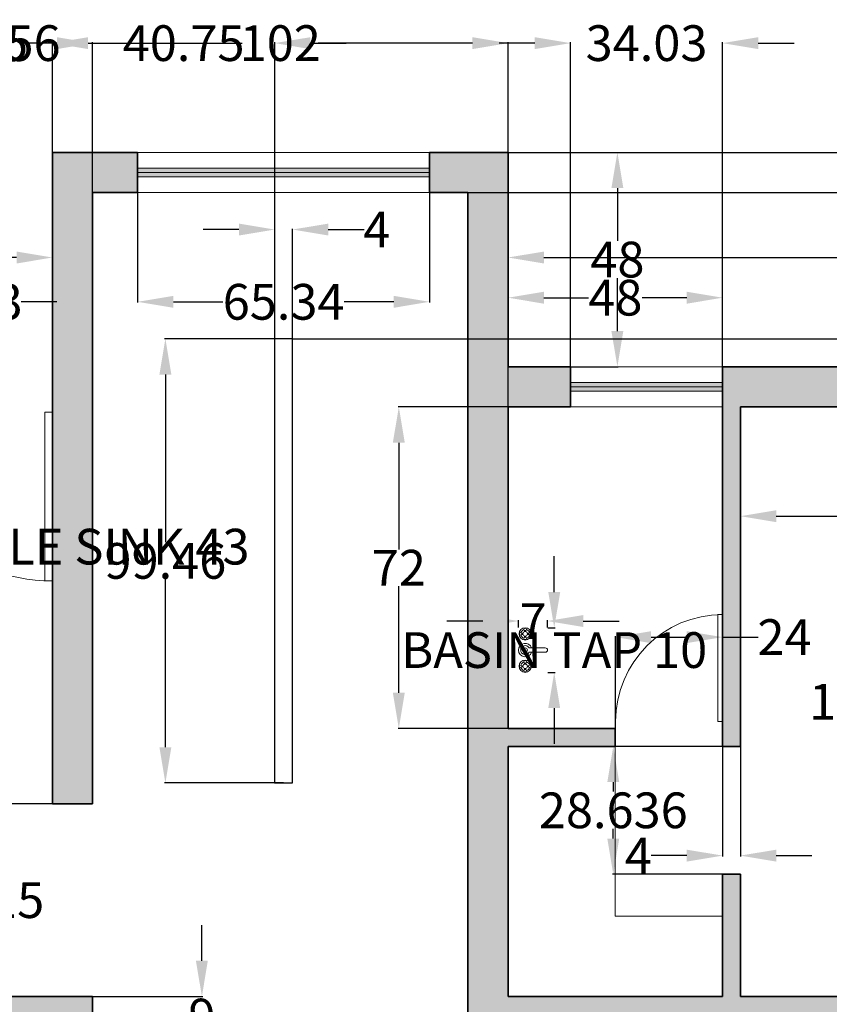
# Model space of a CAD drawing. Units: inches. Extents: x -52 to 678, y 23 to 685.
# Tile 8 of 11: x 249 to 431, y 334 to 555. Entities that reach past the tile are written whole.
import ezdxf

# ---------------------------------------------------------------- set-up
doc = ezdxf.new("R2010")
doc.units = ezdxf.units.IN
doc.header["$MEASUREMENT"] = 0
for name, color, linetype, lineweight in [('A-ANNO-DIMS', 2, 'Continuous', 18), ('A-DOOR', 3, 'Continuous', 18), ('A-FLOR-CASE', 8, 'Continuous', 18), ('A-FLOR-FIXT', 9, 'Continuous', 18), ('A-FLOR-STRS', 7, 'Continuous', 25), ('A-GLAZ', 4, 'Continuous', 18), ('A-WALL', 7, 'Continuous', 35)]:
    doc.layers.add(name, color=color, linetype=linetype, lineweight=lineweight)
doc.layers.add('A-GLAZ-PATT', color=18, linetype='Continuous', lineweight=13, true_color=0x000000)
doc.layers.add('A-WALL-PATT', color=18, linetype='Continuous', lineweight=13, true_color=0x000000)
doc.styles.get("Standard").update_dxf_attribs({"font": 'arial.ttf'})
doc.dimstyles.get("Standard").update_dxf_attribs({"dimtxt": 8, "dimasz": 8, "dimexe": 0.18, "dimexo": 0.0625, "dimgap": 0.09, "dimtad": 0, "dimtih": 1, "dimtoh": 1, "dimdec": 0, "dimzin": 0, "dimdsep": 46, "dimlunit": 3, "dimtxsty": 'Standard', "dimcen": 0.09, "dimadec": 0, "dimazin": 0, "dimtfac": 1, "dimtdec": 0, "dimtofl": 0, "dimtmove": 0, "dimatfit": 3, "dimfxl": 1, "dimtolj": 1, "dimtzin": 0, "dimarcsym": 0})

# ---------------------------------------------------------------- blocks, each defined once
blk = doc.blocks.new('Faucet - Bathroom top')
for p, q in [((-4.107, 0.125), (-4.375, 0.125)), ((-3.75, 0.4788), (-3.75, 0.75)), ((-3.5, 0.482), (-3.5, 0.75)), ((-3.1461, 0.125), (-2.875, 0.125)), ((3.143, 0.125), (2.875, 0.125)), ((3.5, 0.4788), (3.5, 0.75)), ((3.75, 0.482), (3.75, 0.75)), ((4.1039, 0.125), (4.375, 0.125)), ((-4.1039, -0.125), (-4.375, -0.125)), ((-3.75, -0.4821), (-3.75, -0.75)), ((-3.5, -0.4789), (-3.5, -0.75)), ((-3.143, -0.125), (-2.875, -0.125)), ((-0.5, -0.8639), (-0.5, -4.5)), ((0.5, -4.5), (0.5, -0.8631)), ((3.1461, -0.125), (2.875, -0.125)), ((3.5, -0.4821), (3.5, -0.75)), ((3.75, -0.4789), (3.75, -0.75)), ((4.107, -0.125), (4.375, -0.125))]:
    blk.add_line(p, q)
for centre, radius in [((-3.625, 0), 1.375), ((-4.625, 0), 0.2795), ((-3.625, 0), 0.5), ((-3.625, 1), 0.2795), ((-2.625, 0), 0.2795), ((0, 0), 0.5), ((3.625, 0), 1.375), ((2.625, 0), 0.2795), ((3.625, 0), 0.5), ((3.625, 1), 0.2795), ((4.625, 0), 0.2795), ((-3.625, -1), 0.2795), ((3.625, -1), 0.2795)]:
    blk.add_circle(centre, radius)
for centre, radius, start, end in [((-3.625, 0), 1, 105.2407, 164.2093), ((-3.625, 0), 1, 16.44125, 74.07887), ((0, 0), 1.5, 289.6514, 250.3603), ((0, 0), 1, 300.3431, 239.7554), ((3.625, 0), 1, 106.12, 164.0884), ((3.625, 0), 1, 16.23422, 73.90469), ((-3.625, 0), 1, 196.2342, 253.9047), ((-3.625, 0), 1, 286.12, 344.0884), ((3.625, 0), 1, 196.4413, 254.0789), ((3.625, 0), 1, 285.2407, 344.2093), ((0, -4.5), 0.5, 180, 0)]:
    blk.add_arc(centre, radius, start, end)
blk = doc.blocks.new('*U16')
for p, q in [((-40, 0), (-40, 6)), ((0, 0), (0, 6))]:
    blk.add_line(p, q)
blk.add_lwpolyline([(0, 0), (0, -40), (-1.75, -40), (-1.75, 0)], close=True)
blk.add_arc((0, 0), 40, 180, 270)
blk = doc.blocks.new('*U15')
for p, q in [((0, 0), (0, -6)), ((-40, 0), (-40, -6))]:
    blk.add_line(p, q)
blk.add_lwpolyline([(0, 0), (0, 40), (-1.75, 40), (-1.75, 0)], close=True)
blk.add_arc((0, 0), 40, 90, 180)
blk = doc.blocks.new('*D29')
at = {"layer": 'A-ANNO-DIMS', "color": 0, "lineweight": -2, "transparency": 16777216}
for p, q in [((163.02, 443.19), (163.02, 436.67)), ((205.67, 443.19), (205.67, 436.67)), ((171.02, 436.85), (197.67, 436.85)), ((205.67, 436.85), (213.67, 436.85))]:
    blk.add_line(p, q, dxfattribs=at)
at = {"layer": 'A-ANNO-DIMS', "color": 0, "transparency": 16777216}
for points in [[(171.02, 438.19), (171.02, 435.52), (163.02, 436.85)], [(197.67, 438.19), (197.67, 435.52), (205.67, 436.85)]]:
    blk.add_solid(points, dxfattribs=at)
at = {"layer": 'Defpoints', "color": 0, "transparency": 16777216}
for p in [(163.02, 443.25), (205.67, 443.25), (205.67, 436.85)]:
    blk.add_point(p, dxfattribs=at)
at = {"layer": 'A-ANNO-DIMS', "color": 0, "transparency": 16777216, "insert": (258.41, 436.85), "char_height": 8, "attachment_point": 5}
blk.add_mtext('\\A1;DOUBLE SINK 43', dxfattribs=at)
blk = doc.blocks.new('*D35')
at = {"layer": 'A-ANNO-DIMS', "color": 0, "lineweight": -2, "transparency": 16777216}
for p, q in [((368.93, 426.69), (368.93, 434.69)), ((367.5, 418.69), (369.11, 418.69)), ((367.5, 408.69), (369.11, 408.69)), ((368.93, 400.69), (368.93, 392.69))]:
    blk.add_line(p, q, dxfattribs=at)
at = {"layer": 'A-ANNO-DIMS', "color": 0, "transparency": 16777216}
for points in [[(367.6, 426.69), (370.27, 426.69), (368.93, 418.69)], [(367.6, 400.69), (370.27, 400.69), (368.93, 408.69)]]:
    blk.add_solid(points, dxfattribs=at)
at = {"layer": 'Defpoints', "color": 0, "transparency": 16777216}
for p in [(367.43, 418.69), (368.93, 418.69), (367.43, 408.69)]:
    blk.add_point(p, dxfattribs=at)
at = {"layer": 'A-ANNO-DIMS', "color": 0, "transparency": 16777216, "insert": (368.93, 413.69), "char_height": 8, "attachment_point": 5}
blk.add_mtext('\\A1;BASIN TAP 10', dxfattribs=at)
blk = doc.blocks.new('*D36')
at = {"layer": 'A-ANNO-DIMS', "color": 0, "lineweight": -2, "transparency": 16777216}
for p, q in [((352.93, 420.19), (344.93, 420.19)), ((360.93, 418.76), (360.93, 420.37)), ((367.43, 418.76), (367.43, 420.37)), ((375.43, 420.19), (383.43, 420.19))]:
    blk.add_line(p, q, dxfattribs=at)
at = {"layer": 'A-ANNO-DIMS', "color": 0, "transparency": 16777216}
for points in [[(352.93, 421.53), (352.93, 418.86), (360.93, 420.19)], [(375.43, 421.53), (375.43, 418.86), (367.43, 420.19)]]:
    blk.add_solid(points, dxfattribs=at)
at = {"layer": 'Defpoints', "color": 0, "transparency": 16777216}
for p in [(360.93, 420.19), (360.93, 418.69), (367.43, 418.69)]:
    blk.add_point(p, dxfattribs=at)
at = {"layer": 'A-ANNO-DIMS', "color": 0, "transparency": 16777216, "insert": (364.18, 420.19), "char_height": 8, "attachment_point": 5}
blk.add_mtext('\\A1;7', dxfattribs=at)
blk = doc.blocks.new('*D40')
at = {"layer": 'A-ANNO-DIMS', "color": 0, "lineweight": -2, "transparency": 16777216}
for p, q in [((358.67, 525.13), (600.25, 525.13)), ((600.07, 517.13), (600.07, 293.23)), ((600.07, 61.13), (600.07, 285.02)), ((575.67, 53.13), (600.25, 53.13))]:
    blk.add_line(p, q, dxfattribs=at)
at = {"layer": 'A-ANNO-DIMS', "color": 0, "transparency": 16777216}
for points in [[(598.73, 517.13), (601.4, 517.13), (600.07, 525.13)], [(598.73, 61.13), (601.4, 61.13), (600.07, 53.13)]]:
    blk.add_solid(points, dxfattribs=at)
at = {"layer": 'Defpoints', "color": 0, "transparency": 16777216}
for p in [(358.61, 525.13), (600.07, 525.13), (575.61, 53.13)]:
    blk.add_point(p, dxfattribs=at)
at = {"layer": 'A-ANNO-DIMS', "color": 0, "transparency": 16777216, "insert": (600.07, 289.13), "char_height": 8, "attachment_point": 5}
blk.add_mtext('\\A1;472', dxfattribs=at)
blk = doc.blocks.new('*D41')
at = {"layer": 'A-ANNO-DIMS', "color": 0, "lineweight": -2, "transparency": 16777216}
for p, q in [((91.61, 477.19), (91.61, 501.77)), ((99.61, 501.59), (165.52, 501.59)), ((248.61, 501.59), (182.69, 501.59)), ((256.61, 477.19), (256.61, 501.77))]:
    blk.add_line(p, q, dxfattribs=at)
at = {"layer": 'A-ANNO-DIMS', "color": 0, "transparency": 16777216}
for points in [[(99.61, 502.92), (99.61, 500.25), (91.61, 501.59)], [(248.61, 502.92), (248.61, 500.25), (256.61, 501.59)]]:
    blk.add_solid(points, dxfattribs=at)
at = {"layer": 'Defpoints', "color": 0, "transparency": 16777216}
for p in [(256.61, 501.59), (91.61, 477.13), (256.61, 477.13)]:
    blk.add_point(p, dxfattribs=at)
at = {"layer": 'A-ANNO-DIMS', "color": 0, "transparency": 16777216, "insert": (174.11, 501.59), "char_height": 8, "attachment_point": 5}
blk.add_mtext('\\A1;165', dxfattribs=at)
blk = doc.blocks.new('*D42')
at = {"layer": 'A-ANNO-DIMS', "color": 0, "lineweight": -2, "transparency": 16777216}
for p, q in [((256.61, 525.19), (256.61, 549.77)), ((264.61, 549.59), (299.1, 549.59)), ((350.61, 549.59), (316.12, 549.59)), ((358.61, 525.19), (358.61, 549.77))]:
    blk.add_line(p, q, dxfattribs=at)
at = {"layer": 'A-ANNO-DIMS', "color": 0, "transparency": 16777216}
for points in [[(264.61, 550.92), (264.61, 548.25), (256.61, 549.59)], [(350.61, 550.92), (350.61, 548.25), (358.61, 549.59)]]:
    blk.add_solid(points, dxfattribs=at)
at = {"layer": 'Defpoints', "color": 0, "transparency": 16777216}
for p in [(358.61, 549.59), (256.61, 525.13), (358.61, 525.13)]:
    blk.add_point(p, dxfattribs=at)
at = {"layer": 'A-ANNO-DIMS', "color": 0, "transparency": 16777216, "insert": (307.61, 549.59), "char_height": 8, "attachment_point": 5}
blk.add_mtext('\\A1;102', dxfattribs=at)
blk = doc.blocks.new('*D43')
at = {"layer": 'A-ANNO-DIMS', "color": 0, "lineweight": -2, "transparency": 16777216}
for p, q in [((358.61, 477.19), (358.61, 501.77)), ((366.61, 501.59), (458.11, 501.59)), ((567.61, 501.59), (476.1, 501.59)), ((575.61, 477.19), (575.61, 501.77))]:
    blk.add_line(p, q, dxfattribs=at)
at = {"layer": 'A-ANNO-DIMS', "color": 0, "transparency": 16777216}
for points in [[(366.61, 502.92), (366.61, 500.25), (358.61, 501.59)], [(567.61, 502.92), (567.61, 500.25), (575.61, 501.59)]]:
    blk.add_solid(points, dxfattribs=at)
at = {"layer": 'Defpoints', "color": 0, "transparency": 16777216}
for p in [(575.61, 501.59), (358.61, 477.13), (575.61, 477.13)]:
    blk.add_point(p, dxfattribs=at)
at = {"layer": 'A-ANNO-DIMS', "color": 0, "transparency": 16777216, "insert": (467.11, 501.59), "char_height": 8, "attachment_point": 5}
blk.add_mtext('\\A1;217', dxfattribs=at)
blk = doc.blocks.new('*D44')
at = {"layer": 'A-ANNO-DIMS', "color": 0, "lineweight": -2, "transparency": 16777216}
for p, q in [((358.67, 525.13), (383.25, 525.13)), ((383.07, 517.13), (383.07, 505.3)), ((383.07, 485.13), (383.07, 496.95)), ((358.67, 477.13), (383.25, 477.13))]:
    blk.add_line(p, q, dxfattribs=at)
at = {"layer": 'A-ANNO-DIMS', "color": 0, "transparency": 16777216}
for points in [[(381.73, 517.13), (384.4, 517.13), (383.07, 525.13)], [(381.73, 485.13), (384.4, 485.13), (383.07, 477.13)]]:
    blk.add_solid(points, dxfattribs=at)
at = {"layer": 'Defpoints', "color": 0, "transparency": 16777216}
for p in [(358.61, 525.13), (358.61, 477.13), (383.07, 477.13)]:
    blk.add_point(p, dxfattribs=at)
at = {"layer": 'A-ANNO-DIMS', "color": 0, "transparency": 16777216, "insert": (383.07, 501.13), "char_height": 8, "attachment_point": 5}
blk.add_mtext('\\A1;48', dxfattribs=at)
blk = doc.blocks.new('*D53')
at = {"layer": 'A-ANNO-DIMS', "color": 0, "lineweight": -2, "transparency": 16777216}
for p, q in [((358.61, 468.19), (358.61, 492.77)), ((366.61, 492.59), (376.62, 492.59)), ((398.61, 492.59), (388.59, 492.59)), ((406.61, 468.19), (406.61, 492.77))]:
    blk.add_line(p, q, dxfattribs=at)
at = {"layer": 'A-ANNO-DIMS', "color": 0, "transparency": 16777216}
for points in [[(366.61, 493.92), (366.61, 491.25), (358.61, 492.59)], [(398.61, 493.92), (398.61, 491.25), (406.61, 492.59)]]:
    blk.add_solid(points, dxfattribs=at)
at = {"layer": 'Defpoints', "color": 0, "transparency": 16777216}
for p in [(406.61, 492.59), (358.61, 468.13), (406.61, 468.13)]:
    blk.add_point(p, dxfattribs=at)
at = {"layer": 'A-ANNO-DIMS', "color": 0, "transparency": 16777216, "insert": (382.61, 492.59), "char_height": 8, "attachment_point": 5}
blk.add_mtext('\\A1;48', dxfattribs=at)
blk = doc.blocks.new('*D54')
at = {"layer": 'A-ANNO-DIMS', "color": 0, "lineweight": -2, "transparency": 16777216}
for p, q in [((358.54, 468.13), (333.97, 468.13)), ((334.15, 460.13), (334.15, 436.23)), ((334.15, 404.13), (334.15, 428.02)), ((358.54, 396.13), (333.97, 396.13))]:
    blk.add_line(p, q, dxfattribs=at)
at = {"layer": 'A-ANNO-DIMS', "color": 0, "transparency": 16777216}
for points in [[(332.81, 460.13), (335.48, 460.13), (334.15, 468.13)], [(332.81, 404.13), (335.48, 404.13), (334.15, 396.13)]]:
    blk.add_solid(points, dxfattribs=at)
at = {"layer": 'Defpoints', "color": 0, "transparency": 16777216}
for p in [(334.15, 468.13), (358.61, 468.13), (358.61, 396.13)]:
    blk.add_point(p, dxfattribs=at)
at = {"layer": 'A-ANNO-DIMS', "color": 0, "transparency": 16777216, "insert": (334.15, 432.13), "char_height": 8, "attachment_point": 5}
blk.add_mtext('\\A1;72', dxfattribs=at)
blk = doc.blocks.new('*D57')
at = {"layer": 'A-ANNO-DIMS', "color": 0, "lineweight": -2, "transparency": 16777216}
for p, q in [((410.61, 468.06), (410.61, 443.49)), ((566.61, 468.06), (566.61, 443.49)), ((418.61, 443.67), (480.06, 443.67)), ((558.61, 443.67), (497.15, 443.67))]:
    blk.add_line(p, q, dxfattribs=at)
at = {"layer": 'A-ANNO-DIMS', "color": 0, "transparency": 16777216}
for points in [[(418.61, 445), (418.61, 442.33), (410.61, 443.67)], [(558.61, 445), (558.61, 442.33), (566.61, 443.67)]]:
    blk.add_solid(points, dxfattribs=at)
at = {"layer": 'Defpoints', "color": 0, "transparency": 16777216}
for p in [(410.61, 468.13), (566.61, 468.13), (410.61, 443.67)]:
    blk.add_point(p, dxfattribs=at)
at = {"layer": 'A-ANNO-DIMS', "color": 0, "transparency": 16777216, "insert": (488.61, 443.67), "char_height": 8, "attachment_point": 5}
blk.add_mtext('\\A1;156', dxfattribs=at)
blk = doc.blocks.new('*D58')
at = {"layer": 'A-ANNO-DIMS', "color": 0, "lineweight": -2, "transparency": 16777216}
for p, q in [((410.67, 468.13), (435.25, 468.13)), ((435.07, 460.13), (435.07, 406.3)), ((435.07, 344.13), (435.07, 397.95)), ((410.67, 336.13), (435.25, 336.13))]:
    blk.add_line(p, q, dxfattribs=at)
at = {"layer": 'A-ANNO-DIMS', "color": 0, "transparency": 16777216}
for points in [[(433.73, 460.13), (436.4, 460.13), (435.07, 468.13)], [(433.73, 344.13), (436.4, 344.13), (435.07, 336.13)]]:
    blk.add_solid(points, dxfattribs=at)
at = {"layer": 'Defpoints', "color": 0, "transparency": 16777216}
for p in [(410.61, 468.13), (410.61, 336.13), (435.07, 336.13)]:
    blk.add_point(p, dxfattribs=at)
at = {"layer": 'A-ANNO-DIMS', "color": 0, "transparency": 16777216, "insert": (435.07, 402.13), "char_height": 8, "attachment_point": 5}
blk.add_mtext('\\A1;132', dxfattribs=at)
blk = doc.blocks.new('*D59')
at = {"layer": 'A-ANNO-DIMS', "color": 0, "lineweight": -2, "transparency": 16777216}
for p, q in [((290.07, 344.13), (290.07, 352.13)), ((265.67, 336.13), (290.25, 336.13)), ((265.67, 327.13), (290.25, 327.13)), ((290.07, 319.13), (290.07, 311.13))]:
    blk.add_line(p, q, dxfattribs=at)
at = {"layer": 'A-ANNO-DIMS', "color": 0, "transparency": 16777216}
for points in [[(288.73, 344.13), (291.4, 344.13), (290.07, 336.13)], [(288.73, 319.13), (291.4, 319.13), (290.07, 327.13)]]:
    blk.add_solid(points, dxfattribs=at)
at = {"layer": 'Defpoints', "color": 0, "transparency": 16777216}
for p in [(265.61, 336.13), (265.61, 327.13), (290.07, 327.13)]:
    blk.add_point(p, dxfattribs=at)
at = {"layer": 'A-ANNO-DIMS', "color": 0, "transparency": 16777216, "insert": (290.07, 331.63), "char_height": 8, "attachment_point": 5}
blk.add_mtext('\\A1;9', dxfattribs=at)
blk = doc.blocks.new('*D60')
at = {"layer": 'A-ANNO-DIMS', "color": 0, "lineweight": -2, "transparency": 16777216}
for p, q in [((406.61, 392.06), (406.61, 367.49)), ((410.61, 392.06), (410.61, 367.49)), ((398.61, 367.67), (390.61, 367.67)), ((418.61, 367.67), (426.61, 367.67))]:
    blk.add_line(p, q, dxfattribs=at)
at = {"layer": 'A-ANNO-DIMS', "color": 0, "transparency": 16777216}
for points in [[(398.61, 369), (398.61, 366.33), (406.61, 367.67)], [(418.61, 369), (418.61, 366.33), (410.61, 367.67)]]:
    blk.add_solid(points, dxfattribs=at)
at = {"layer": 'Defpoints', "color": 0, "transparency": 16777216}
for p in [(406.61, 392.13), (410.61, 392.13), (406.61, 367.67)]:
    blk.add_point(p, dxfattribs=at)
at = {"layer": 'A-ANNO-DIMS', "color": 0, "transparency": 16777216, "insert": (387.75, 367.67), "char_height": 8, "attachment_point": 5}
blk.add_mtext('\\A1;4', dxfattribs=at)
blk = doc.blocks.new('*D61')
at = {"layer": 'A-ANNO-DIMS', "color": 0, "lineweight": -2, "transparency": 16777216}
for p, q in [((210.46, 549.59), (202.46, 549.59)), ((218.46, 477.19), (218.46, 549.77)), ((256.61, 477.19), (256.61, 549.77)), ((264.61, 549.59), (272.61, 549.59))]:
    blk.add_line(p, q, dxfattribs=at)
at = {"layer": 'A-ANNO-DIMS', "color": 0, "transparency": 16777216}
for points in [[(210.46, 550.92), (210.46, 548.25), (218.46, 549.59)], [(264.61, 550.92), (264.61, 548.25), (256.61, 549.59)]]:
    blk.add_solid(points, dxfattribs=at)
at = {"layer": 'Defpoints', "color": 0, "transparency": 16777216}
for p in [(256.61, 549.59), (218.46, 477.13), (256.61, 477.13)]:
    blk.add_point(p, dxfattribs=at)
at = {"layer": 'A-ANNO-DIMS', "color": 0, "transparency": 16777216, "insert": (237.53, 549.59), "char_height": 8, "attachment_point": 5}
blk.add_mtext('\\A1;38.15', dxfattribs=at)
blk = doc.blocks.new('*D64')
at = {"layer": 'A-ANNO-DIMS', "color": 0, "lineweight": -2, "transparency": 16777216}
for p, q in [((275.69, 516.06), (275.69, 491.49)), ((341.02, 516.06), (341.02, 491.49)), ((283.69, 491.67), (294.76, 491.67)), ((333.02, 491.67), (321.95, 491.67))]:
    blk.add_line(p, q, dxfattribs=at)
at = {"layer": 'A-ANNO-DIMS', "color": 0, "transparency": 16777216}
for points in [[(283.69, 493), (283.69, 490.33), (275.69, 491.67)], [(333.02, 493), (333.02, 490.33), (341.02, 491.67)]]:
    blk.add_solid(points, dxfattribs=at)
at = {"layer": 'Defpoints', "color": 0, "transparency": 16777216}
for p in [(275.69, 516.13), (341.02, 516.13), (275.69, 491.67)]:
    blk.add_point(p, dxfattribs=at)
at = {"layer": 'A-ANNO-DIMS', "color": 0, "transparency": 16777216, "insert": (308.36, 491.67), "char_height": 8, "attachment_point": 5}
blk.add_mtext('\\A1;65.34', dxfattribs=at)
blk = doc.blocks.new('*D65')
at = {"layer": 'A-ANNO-DIMS', "color": 0, "lineweight": -2, "transparency": 16777216}
for p, q in [((265.61, 516.06), (265.61, 491.49)), ((275.69, 516.06), (275.69, 491.49)), ((257.61, 491.67), (249.61, 491.67)), ((283.69, 491.67), (291.69, 491.67))]:
    blk.add_line(p, q, dxfattribs=at)
at = {"layer": 'A-ANNO-DIMS', "color": 0, "transparency": 16777216}
for points in [[(257.61, 493), (257.61, 490.33), (265.61, 491.67)], [(283.69, 493), (283.69, 490.33), (275.69, 491.67)]]:
    blk.add_solid(points, dxfattribs=at)
at = {"layer": 'Defpoints', "color": 0, "transparency": 16777216}
for p in [(265.61, 516.13), (275.69, 516.13), (265.61, 491.67)]:
    blk.add_point(p, dxfattribs=at)
at = {"layer": 'A-ANNO-DIMS', "color": 0, "transparency": 16777216, "insert": (233.29, 491.67), "char_height": 8, "attachment_point": 5}
blk.add_mtext('\\A1;10.083', dxfattribs=at)
blk = doc.blocks.new('*D68')
at = {"layer": 'A-ANNO-DIMS', "color": 0, "lineweight": -2, "transparency": 16777216}
for p, q in [((364.58, 549.59), (356.58, 549.59)), ((372.58, 477.19), (372.58, 549.77)), ((406.61, 477.19), (406.61, 549.77)), ((414.61, 549.59), (422.61, 549.59))]:
    blk.add_line(p, q, dxfattribs=at)
at = {"layer": 'A-ANNO-DIMS', "color": 0, "transparency": 16777216}
for points in [[(364.58, 550.92), (364.58, 548.25), (372.58, 549.59)], [(414.61, 550.92), (414.61, 548.25), (406.61, 549.59)]]:
    blk.add_solid(points, dxfattribs=at)
at = {"layer": 'Defpoints', "color": 0, "transparency": 16777216}
for p in [(406.61, 549.59), (372.58, 477.13), (406.61, 477.13)]:
    blk.add_point(p, dxfattribs=at)
at = {"layer": 'A-ANNO-DIMS', "color": 0, "transparency": 16777216, "insert": (389.59, 549.59), "char_height": 8, "attachment_point": 5}
blk.add_mtext('\\A1;34.03', dxfattribs=at)
blk = doc.blocks.new('*D81')
at = {"layer": 'A-ANNO-DIMS', "color": 0, "lineweight": -2, "transparency": 16777216}
for p, q in [((306.29, 483.39), (281.72, 483.39)), ((281.9, 475.39), (281.9, 437.84)), ((281.9, 391.93), (281.9, 429.49)), ((306.29, 383.93), (281.72, 383.93))]:
    blk.add_line(p, q, dxfattribs=at)
at = {"layer": 'A-ANNO-DIMS', "color": 0, "transparency": 16777216}
for points in [[(280.56, 475.39), (283.23, 475.39), (281.9, 483.39)], [(280.56, 391.93), (283.23, 391.93), (281.9, 383.93)]]:
    blk.add_solid(points, dxfattribs=at)
at = {"layer": 'Defpoints', "color": 0, "transparency": 16777216}
for p in [(281.9, 483.39), (306.36, 483.39), (306.36, 383.93)]:
    blk.add_point(p, dxfattribs=at)
at = {"layer": 'A-ANNO-DIMS', "color": 0, "transparency": 16777216, "insert": (281.9, 433.66), "char_height": 8, "attachment_point": 5}
blk.add_mtext('\\A1;99.46', dxfattribs=at)
blk = doc.blocks.new('*D82')
at = {"layer": 'A-ANNO-DIMS', "color": 0, "lineweight": -2, "transparency": 16777216}
for p, q in [((298.36, 507.85), (290.36, 507.85)), ((306.36, 483.45), (306.36, 508.03)), ((310.36, 483.45), (310.36, 508.03)), ((318.36, 507.85), (326.36, 507.85))]:
    blk.add_line(p, q, dxfattribs=at)
at = {"layer": 'A-ANNO-DIMS', "color": 0, "transparency": 16777216}
for points in [[(298.36, 509.18), (298.36, 506.52), (306.36, 507.85)], [(318.36, 509.18), (318.36, 506.52), (310.36, 507.85)]]:
    blk.add_solid(points, dxfattribs=at)
at = {"layer": 'Defpoints', "color": 0, "transparency": 16777216}
for p in [(310.36, 507.85), (306.36, 483.39), (310.36, 483.39)]:
    blk.add_point(p, dxfattribs=at)
at = {"layer": 'A-ANNO-DIMS', "color": 0, "transparency": 16777216, "insert": (329.21, 507.85), "char_height": 8, "attachment_point": 5}
blk.add_mtext('\\A1;4', dxfattribs=at)
blk = doc.blocks.new('*D83')
at = {"layer": 'A-ANNO-DIMS', "color": 0, "lineweight": -2, "transparency": 16777216}
for p, q in [((257.61, 549.59), (249.61, 549.59)), ((265.61, 379.34), (265.61, 549.77)), ((306.36, 383.99), (306.36, 549.77)), ((314.36, 549.59), (322.36, 549.59))]:
    blk.add_line(p, q, dxfattribs=at)
at = {"layer": 'A-ANNO-DIMS', "color": 0, "transparency": 16777216}
for points in [[(257.61, 550.92), (257.61, 548.25), (265.61, 549.59)], [(314.36, 550.92), (314.36, 548.25), (306.36, 549.59)]]:
    blk.add_solid(points, dxfattribs=at)
at = {"layer": 'Defpoints', "color": 0, "transparency": 16777216}
for p in [(306.36, 549.59), (306.36, 383.93), (265.61, 379.27)]:
    blk.add_point(p, dxfattribs=at)
at = {"layer": 'A-ANNO-DIMS', "color": 0, "transparency": 16777216, "insert": (285.98, 549.59), "char_height": 8, "attachment_point": 5}
blk.add_mtext('\\A1;40.75', dxfattribs=at)
blk = doc.blocks.new('*D84')
at = {"layer": 'A-ANNO-DIMS', "color": 0, "lineweight": -2, "transparency": 16777216}
for p, q in [((265.54, 379.27), (240.97, 379.27)), ((241.15, 371.27), (241.15, 361.88)), ((241.15, 344.13), (241.15, 353.52)), ((265.54, 336.13), (240.97, 336.13))]:
    blk.add_line(p, q, dxfattribs=at)
at = {"layer": 'A-ANNO-DIMS', "color": 0, "transparency": 16777216}
for points in [[(239.81, 371.27), (242.48, 371.27), (241.15, 379.27)], [(239.81, 344.13), (242.48, 344.13), (241.15, 336.13)]]:
    blk.add_solid(points, dxfattribs=at)
at = {"layer": 'Defpoints', "color": 0, "transparency": 16777216}
for p in [(241.15, 379.27), (265.61, 379.27), (265.61, 336.13)]:
    blk.add_point(p, dxfattribs=at)
at = {"layer": 'A-ANNO-DIMS', "color": 0, "transparency": 16777216, "insert": (241.15, 357.7), "char_height": 8, "attachment_point": 5}
blk.add_mtext('\\A1;43.15', dxfattribs=at)
blk = doc.blocks.new('*D85')
at = {"layer": 'A-ANNO-DIMS', "color": 0, "lineweight": -2, "transparency": 16777216}
for p, q in [((349.67, 516.13), (600.25, 516.13)), ((600.07, 508.13), (600.07, 503.94)), ((600.07, 491.39), (600.07, 495.58)), ((310.42, 483.39), (600.25, 483.39))]:
    blk.add_line(p, q, dxfattribs=at)
at = {"layer": 'A-ANNO-DIMS', "color": 0, "transparency": 16777216}
for points in [[(598.73, 508.13), (601.4, 508.13), (600.07, 516.13)], [(598.73, 491.39), (601.4, 491.39), (600.07, 483.39)]]:
    blk.add_solid(points, dxfattribs=at)
at = {"layer": 'Defpoints', "color": 0, "transparency": 16777216}
for p in [(349.61, 516.13), (600.07, 516.13), (310.36, 483.39)]:
    blk.add_point(p, dxfattribs=at)
at = {"layer": 'A-ANNO-DIMS', "color": 0, "transparency": 16777216, "insert": (600.07, 499.76), "char_height": 8, "attachment_point": 5}
blk.add_mtext('\\A1;32.736', dxfattribs=at)
blk = doc.blocks.new('*D86')
at = {"layer": 'A-ANNO-DIMS', "color": 0, "lineweight": -2, "transparency": 16777216}
for p, q in [((382.61, 392.19), (382.61, 416.77)), ((406.61, 392.19), (406.61, 416.77)), ((390.61, 416.59), (398.61, 416.59)), ((406.61, 416.59), (414.61, 416.59))]:
    blk.add_line(p, q, dxfattribs=at)
at = {"layer": 'A-ANNO-DIMS', "color": 0, "transparency": 16777216}
for points in [[(390.61, 417.92), (390.61, 415.25), (382.61, 416.59)], [(398.61, 417.92), (398.61, 415.25), (406.61, 416.59)]]:
    blk.add_solid(points, dxfattribs=at)
at = {"layer": 'Defpoints', "color": 0, "transparency": 16777216}
for p in [(406.61, 416.59), (382.61, 392.13), (406.61, 392.13)]:
    blk.add_point(p, dxfattribs=at)
at = {"layer": 'A-ANNO-DIMS', "color": 0, "transparency": 16777216, "insert": (420.48, 416.59), "char_height": 8, "attachment_point": 5}
blk.add_mtext('\\A1;24', dxfattribs=at)
blk = doc.blocks.new('*D87')
at = {"layer": 'A-ANNO-DIMS', "color": 0, "lineweight": -2, "transparency": 16777216}
for p, q in [((406.54, 392.13), (381.97, 392.13)), ((382.15, 384.13), (382.15, 381.99)), ((382.15, 371.49), (382.15, 373.63)), ((406.54, 363.49), (381.97, 363.49))]:
    blk.add_line(p, q, dxfattribs=at)
at = {"layer": 'A-ANNO-DIMS', "color": 0, "transparency": 16777216}
for points in [[(380.81, 384.13), (383.48, 384.13), (382.15, 392.13)], [(380.81, 371.49), (383.48, 371.49), (382.15, 363.49)]]:
    blk.add_solid(points, dxfattribs=at)
at = {"layer": 'Defpoints', "color": 0, "transparency": 16777216}
for p in [(382.15, 392.13), (406.61, 392.13), (406.61, 363.49)]:
    blk.add_point(p, dxfattribs=at)
at = {"layer": 'A-ANNO-DIMS', "color": 0, "transparency": 16777216, "insert": (382.15, 377.81), "char_height": 8, "attachment_point": 5}
blk.add_mtext('\\A1;28.636', dxfattribs=at)
blk = doc.blocks.new('*D103')
at = {"layer": 'A-ANNO-DIMS', "color": 0, "lineweight": -2, "transparency": 16777216}
for p, q in [((197.61, 266.24), (197.61, 549.77)), ((205.61, 549.59), (209.46, 549.59)), ((217.46, 271.45), (217.46, 549.77)), ((217.46, 549.59), (225.46, 549.59))]:
    blk.add_line(p, q, dxfattribs=at)
at = {"layer": 'A-ANNO-DIMS', "color": 0, "transparency": 16777216}
for points in [[(205.61, 550.92), (205.61, 548.25), (197.61, 549.59)], [(209.46, 550.92), (209.46, 548.25), (217.46, 549.59)]]:
    blk.add_solid(points, dxfattribs=at)
at = {"layer": 'Defpoints', "color": 0, "transparency": 16777216}
for p in [(217.46, 549.59), (217.46, 271.39), (197.61, 266.17)]:
    blk.add_point(p, dxfattribs=at)
at = {"layer": 'A-ANNO-DIMS', "color": 0, "transparency": 16777216, "insert": (241.78, 549.59), "char_height": 8, "attachment_point": 5}
blk.add_mtext('\\A1;19.856', dxfattribs=at)

msp = doc.modelspace()

# ---------------------------------------------------------------- hatches: boundary and pattern name
at = {"layer": 'A-GLAZ-PATT'}
h = msp.add_hatch(color=256, dxfattribs=at)
h.dxf.hatch_style = 1
h.paths.add_polyline_path([(275.688, 521.6267), (275.688, 520.6267), (341.0247, 520.6267), (341.0247, 521.6267)])
h = msp.add_hatch(color=256, dxfattribs=at)
h.dxf.hatch_style = 1
h.paths.add_polyline_path([(341.0247, 519.6267), (341.0247, 520.6267), (275.688, 520.6267), (275.688, 519.6267)])
h = msp.add_hatch(color=256, dxfattribs=at)
h.dxf.hatch_style = 1
h.paths.add_polyline_path([(406.6053, 472.6267), (406.6053, 473.6267), (372.5751, 473.6267), (372.5751, 472.6267)])
h = msp.add_hatch(color=256, dxfattribs=at)
h.dxf.hatch_style = 1
h.paths.add_polyline_path([(372.5751, 472.6267), (372.5751, 471.6267), (406.6053, 471.6267), (406.6053, 472.6267)])
at = {"layer": 'A-WALL-PATT'}
h = msp.add_hatch(color=256, dxfattribs=at)
h.dxf.hatch_style = 1
h.paths.add_polyline_path([(265.6053, 516.1267), (275.688, 516.1267), (275.688, 525.1267), (256.6053, 525.1267), (256.6053, 477.1267), (256.6053, 468.1267), (256.6053, 379.2738), (265.6053, 379.2738)])
h = msp.add_hatch(color=256, dxfattribs=at)
h.dxf.hatch_style = 1
h.paths.add_polyline_path([(349.6053, 340.107), (349.6053, 327.1267), (410.6053, 327.1267), (434.6053, 327.1267), (434.6053, 336.1267), (410.6053, 336.1267), (410.6053, 340.107), (410.6053, 363.4905), (406.6053, 363.4905), (406.6053, 340.107), (406.6053, 336.1267), (358.6053, 336.1267), (358.6053, 340.107), (358.6053, 392.1267), (382.6053, 392.1267), (382.6053, 396.1267), (358.6053, 396.1267), (358.6053, 468.1267), (372.5751, 468.1267), (372.5751, 477.1267), (358.6053, 477.1267), (358.6053, 525.1267), (341.0247, 525.1267), (341.0247, 516.1267), (349.6053, 516.1267)])
h = msp.add_hatch(color=256, dxfattribs=at)
h.dxf.hatch_style = 1
h.paths.add_polyline_path([(410.6053, 477.1267), (406.6053, 477.1267), (406.6053, 392.1267), (410.6053, 392.1267), (410.6053, 468.1267), (454.1942, 468.1267), (454.1942, 477.1267)])
h = msp.add_hatch(color=256, dxfattribs=at)
h.dxf.hatch_style = 1
h.paths.add_polyline_path([(265.6053, 327.1267), (265.6053, 336.1267), (170.301, 336.1267), (170.301, 327.1267)])

# ---------------------------------------------------------------- linework, layer by layer
at = {"layer": 'A-FLOR-CASE'}
for p, q in [((382.6053, 392.1267), (382.6053, 354.0872)), ((382.6053, 354.0872), (406.6053, 354.0872))]:
    msp.add_line(p, q, dxfattribs=at)
at = {"layer": 'A-FLOR-STRS'}
for p, q in [((310.3563, 483.3905), (306.3563, 483.3905)), ((306.3563, 483.3905), (306.3563, 383.9324)), ((310.3563, 383.9324), (310.3563, 483.3905)), ((308.3563, 383.9324), (306.3563, 383.9324)), ((306.3563, 383.9324), (310.3563, 383.9324))]:
    msp.add_line(p, q, dxfattribs=at)
at = {"layer": 'A-GLAZ'}
for p, q in [((275.688, 525.1267), (341.0247, 525.1267)), ((275.688, 521.6267), (341.0247, 521.6267)), ((275.688, 520.6267), (341.0247, 520.6267)), ((275.688, 519.6267), (341.0247, 519.6267)), ((275.688, 516.1267), (341.0247, 516.1267)), ((372.5751, 477.1267), (406.6053, 477.1267)), ((372.5751, 473.6267), (406.6053, 473.6267)), ((372.5751, 472.6267), (406.6053, 472.6267)), ((372.5751, 471.6267), (406.6053, 471.6267)), ((372.5751, 468.1267), (406.6053, 468.1267))]:
    msp.add_line(p, q, dxfattribs=at)
at = {"layer": 'A-WALL'}
for p, q in [((256.6053, 525.1267), (275.688, 525.1267)), ((256.6053, 525.1267), (256.6053, 477.1267)), ((275.688, 525.1267), (256.6053, 525.1267)), ((275.688, 516.1267), (275.688, 525.1267)), ((358.6053, 525.1267), (341.0247, 525.1267)), ((341.0247, 516.1267), (341.0247, 525.1267)), ((341.0247, 525.1267), (358.6053, 525.1267)), ((358.6053, 525.1267), (358.6053, 477.1267)), ((265.6053, 516.1267), (265.6053, 379.2738)), ((275.688, 516.1267), (265.6053, 516.1267)), ((349.6053, 516.1267), (341.0247, 516.1267)), ((349.6053, 516.1267), (349.6053, 340.107)), ((256.6053, 468.1267), (256.6053, 477.1267)), ((372.5751, 477.1267), (358.6053, 477.1267)), ((372.5751, 468.1267), (372.5751, 477.1267)), ((406.6053, 477.1267), (406.6053, 392.1267)), ((410.6053, 477.1267), (406.6053, 477.1267)), ((410.6053, 477.1267), (454.1942, 477.1267)), ((256.6053, 468.1267), (256.6053, 379.2738)), ((372.5751, 468.1267), (358.6053, 468.1267)), ((358.6053, 468.1267), (358.6053, 396.1267)), ((410.6053, 468.1267), (410.6053, 392.1267)), ((410.6053, 468.1267), (454.1942, 468.1267)), ((382.6053, 396.1267), (358.6053, 396.1267)), ((382.6053, 396.1267), (382.6053, 392.1267)), ((382.6053, 392.1267), (358.6053, 392.1267)), ((358.6053, 392.1267), (358.6053, 340.107)), ((410.6053, 392.1267), (406.6053, 392.1267)), ((265.6053, 379.2738), (256.6053, 379.2738)), ((406.6053, 363.4905), (410.6053, 363.4905)), ((406.6053, 363.4905), (406.6053, 340.107)), ((410.6053, 363.4905), (410.6053, 340.107)), ((349.6053, 340.107), (349.6053, 327.1267)), ((358.6053, 336.1267), (358.6053, 340.107)), ((406.6053, 340.107), (406.6053, 336.1267)), ((410.6053, 340.107), (410.6053, 336.1267)), ((170.301, 336.1267), (265.6053, 336.1267)), ((265.6053, 336.1267), (265.6053, 327.1267)), ((406.6053, 336.1267), (358.6053, 336.1267)), ((410.6053, 336.1267), (434.6053, 336.1267))]:
    msp.add_line(p, q, dxfattribs=at)

# ---------------------------------------------------------------- block references
at = {"layer": 'A-DOOR'}
for name, p, xscale, yscale, zscale in [('*U16', (256.6053, 466.957), 0.9449538553603543, 0.9449538553603543, 0.9449538553603543), ('*U15', (406.6053, 397.7156), 0.59813756145571, 0.59813756145571, 0.59813756145571)]:
    msp.add_blockref(name, p, dxfattribs=dict(at, xscale=xscale, yscale=yscale, zscale=zscale))
at = {"layer": 'A-FLOR-FIXT', "rotation": 90}
msp.add_blockref('Faucet - Bathroom top', (362.4344, 413.693), dxfattribs=at)

# ---------------------------------------------------------------- dimensions: what is measured, and where the dimension line sits
at = {"layer": 'A-ANNO-DIMS'}
for base, p1, p2, override, picture, middle in [((217.4609, 549.5867), (197.6053, 266.1726), (217.4609, 271.3879), {"dimdec": 3, "dimlfac": 1, "dimrnd": 0, "dimzin": 0, "dimdsep": 46, "dimlunit": 2}, '*D103', (241.7774, 549.5867)), ((256.6053, 549.5867), (218.4552, 477.1267), (256.6053, 477.1267), {"dimdec": 2, "dimlfac": 1, "dimrnd": 0, "dimzin": 0, "dimdsep": 46, "dimlunit": 2}, '*D61', (237.5302, 549.5867)), ((306.3563, 549.5867), (265.6053, 379.2738), (306.3563, 383.9324), {"dimdec": 2, "dimlfac": 1, "dimrnd": 0, "dimzin": 0, "dimdsep": 46, "dimlunit": 2}, '*D83', (285.9808, 549.5867)), ((358.6053, 549.5867), (256.6053, 525.1267), (358.6053, 525.1267), {"dimdec": 0, "dimlfac": 1, "dimrnd": 0, "dimzin": 0, "dimdsep": 46, "dimlunit": 2}, '*D42', (307.6053, 549.5867)), ((406.6053, 549.5867), (372.5751, 477.1267), (406.6053, 477.1267), {"dimdec": 2, "dimlfac": 1, "dimrnd": 0, "dimzin": 0, "dimdsep": 46, "dimlunit": 2}, '*D68', (389.5902, 549.5867)), ((310.3563, 507.8505), (306.3563, 483.3905), (310.3563, 483.3905), {"dimdec": 0, "dimlfac": 1, "dimrnd": 0, "dimzin": 0, "dimdsep": 46, "dimlunit": 2}, '*D82', (329.213, 507.8505)), ((575.6053, 501.5867), (358.6053, 477.1267), (575.6053, 477.1267), {"dimdec": 0, "dimlfac": 1, "dimrnd": 0, "dimzin": 0, "dimdsep": 46, "dimlunit": 2}, '*D43', (467.1053, 501.5867)), ((406.6053, 492.5867), (358.6053, 468.1267), (406.6053, 468.1267), {"dimdec": 0, "dimlfac": 1, "dimrnd": 0, "dimzin": 0, "dimdsep": 46, "dimlunit": 2}, '*D53', (382.6053, 492.5867)), ((406.6053, 416.5867), (382.6053, 392.1267), (406.6053, 392.1267), {"dimdec": 0, "dimlfac": 1, "dimrnd": 0, "dimzin": 0, "dimdsep": 46, "dimlunit": 2}, '*D86', (420.477, 416.5867))]:
    dim = msp.add_linear_dim(base=base, p1=p1, p2=p2, dimstyle='Standard', override=override, dxfattribs=at)
    dim.commit()
    dim.dimension.update_dxf_attribs({"geometry": picture, "text_midpoint": middle})
for base, p1, p2, angle, override, picture, middle in [((600.0653, 525.1267), (575.6053, 53.1267), (358.6053, 525.1267), 90, {"dimdec": 0, "dimlfac": 1, "dimrnd": 0, "dimzin": 0, "dimdsep": 46, "dimlunit": 2}, '*D40', (600.0653, 289.1267)), ((383.0653, 477.1267), (358.6053, 525.1267), (358.6053, 477.1267), 270, {"dimdec": 0, "dimlfac": 1, "dimrnd": 0, "dimzin": 0, "dimdsep": 46, "dimlunit": 2}, '*D44', (383.0653, 501.1267)), ((265.6053, 491.6667), (275.688, 516.1267), (265.6053, 516.1267), 180, {"dimdec": 3, "dimlfac": 1, "dimrnd": 0, "dimzin": 0, "dimdsep": 46, "dimlunit": 2}, '*D65', (233.2861, 491.6667)), ((275.688, 491.6667), (341.0247, 516.1267), (275.688, 516.1267), 180, {"dimdec": 2, "dimlfac": 1, "dimrnd": 0, "dimzin": 0, "dimdsep": 46, "dimlunit": 2}, '*D64', (308.3563, 491.6667)), ((600.0653, 516.1267), (310.3563, 483.3905), (349.6053, 516.1267), 90, {"dimdec": 3, "dimlfac": 1, "dimrnd": 0, "dimzin": 0, "dimdsep": 46, "dimlunit": 2}, '*D85', (600.0653, 499.7586)), ((256.6053, 501.5867), (91.6053, 477.1267), (256.6053, 477.1267), 0, {"dimdec": 0, "dimlfac": 1, "dimrnd": 0, "dimzin": 0, "dimdsep": 46, "dimlunit": 2}, '*D41', (174.1053, 501.5867)), ((281.8963, 483.3905), (306.3563, 383.9324), (306.3563, 483.3905), 90, {"dimdec": 2, "dimlfac": 1, "dimrnd": 0, "dimzin": 0, "dimdsep": 46, "dimlunit": 2}, '*D81', (281.8963, 433.6614)), ((334.1453, 468.1267), (358.6053, 396.1267), (358.6053, 468.1267), 90, {"dimdec": 0, "dimlfac": 1, "dimrnd": 0, "dimzin": 0, "dimdsep": 46, "dimlunit": 2}, '*D54', (334.1453, 432.1267)), ((410.6053, 443.6667), (566.6053, 468.1267), (410.6053, 468.1267), 180, {"dimdec": 0, "dimlfac": 1, "dimrnd": 0, "dimzin": 0, "dimdsep": 46, "dimlunit": 2}, '*D57', (488.6053, 443.6667)), ((435.0653, 336.1267), (410.6053, 468.1267), (410.6053, 336.1267), 270, {"dimdec": 0, "dimlfac": 1, "dimrnd": 0, "dimzin": 0, "dimdsep": 46, "dimlunit": 2}, '*D58', (435.0653, 402.1267)), ((360.9343, 420.193), (367.4344, 418.693), (360.9343, 418.693), 180, {"dimdec": 0, "dimlfac": 1, "dimrnd": 0, "dimzin": 0, "dimdsep": 46, "dimlunit": 2}, '*D36', (364.1843, 420.193)), ((382.1453, 392.1267), (406.6053, 363.4905), (406.6053, 392.1267), 90, {"dimdec": 3, "dimlfac": 1, "dimrnd": 0, "dimzin": 0, "dimdsep": 46, "dimlunit": 2}, '*D87', (382.1453, 377.8086)), ((406.6053, 367.6667), (410.6053, 392.1267), (406.6053, 392.1267), 180, {"dimdec": 0, "dimlfac": 1, "dimrnd": 0, "dimzin": 0, "dimdsep": 46, "dimlunit": 2}, '*D60', (387.7485, 367.6667)), ((241.1453, 379.2738), (265.6053, 336.1267), (265.6053, 379.2738), 90, {"dimdec": 2, "dimlfac": 1, "dimrnd": 0, "dimzin": 0, "dimdsep": 46, "dimlunit": 2}, '*D84', (241.1453, 357.7003)), ((290.0653, 327.1267), (265.6053, 336.1267), (265.6053, 327.1267), 270, {"dimdec": 0, "dimlfac": 1, "dimrnd": 0, "dimzin": 0, "dimdsep": 46, "dimlunit": 2}, '*D59', (290.0653, 331.6267))]:
    dim = msp.add_linear_dim(base=base, p1=p1, p2=p2, angle=angle, dimstyle='Standard', override=override, dxfattribs=at)
    dim.commit()
    dim.dimension.update_dxf_attribs({"geometry": picture, "text_midpoint": middle})
dim = msp.add_linear_dim(base=(205.6665, 436.854), p1=(163.0219, 443.2507), p2=(205.6665, 443.2507), text='DOUBLE SINK <>', dimstyle='Standard', override={"dimdec": 0, "dimlfac": 1, "dimrnd": 0, "dimzin": 0, "dimdsep": 46, "dimlunit": 2}, dxfattribs=at)
dim.commit()
dim.dimension.update_dxf_attribs({"geometry": '*D29', "text_midpoint": (258.4141, 436.854)})
dim = msp.add_linear_dim(base=(368.9344, 418.693), p1=(367.4344, 408.693), p2=(367.4344, 418.693), angle=90, text='BASIN TAP <>', dimstyle='Standard', override={"dimdec": 0, "dimlfac": 1, "dimrnd": 0, "dimzin": 0, "dimdsep": 46, "dimlunit": 2}, dxfattribs=at)
dim.commit()
dim.dimension.update_dxf_attribs({"geometry": '*D35', "text_midpoint": (368.9344, 413.693)})

doc.saveas('drawing.dxf')
